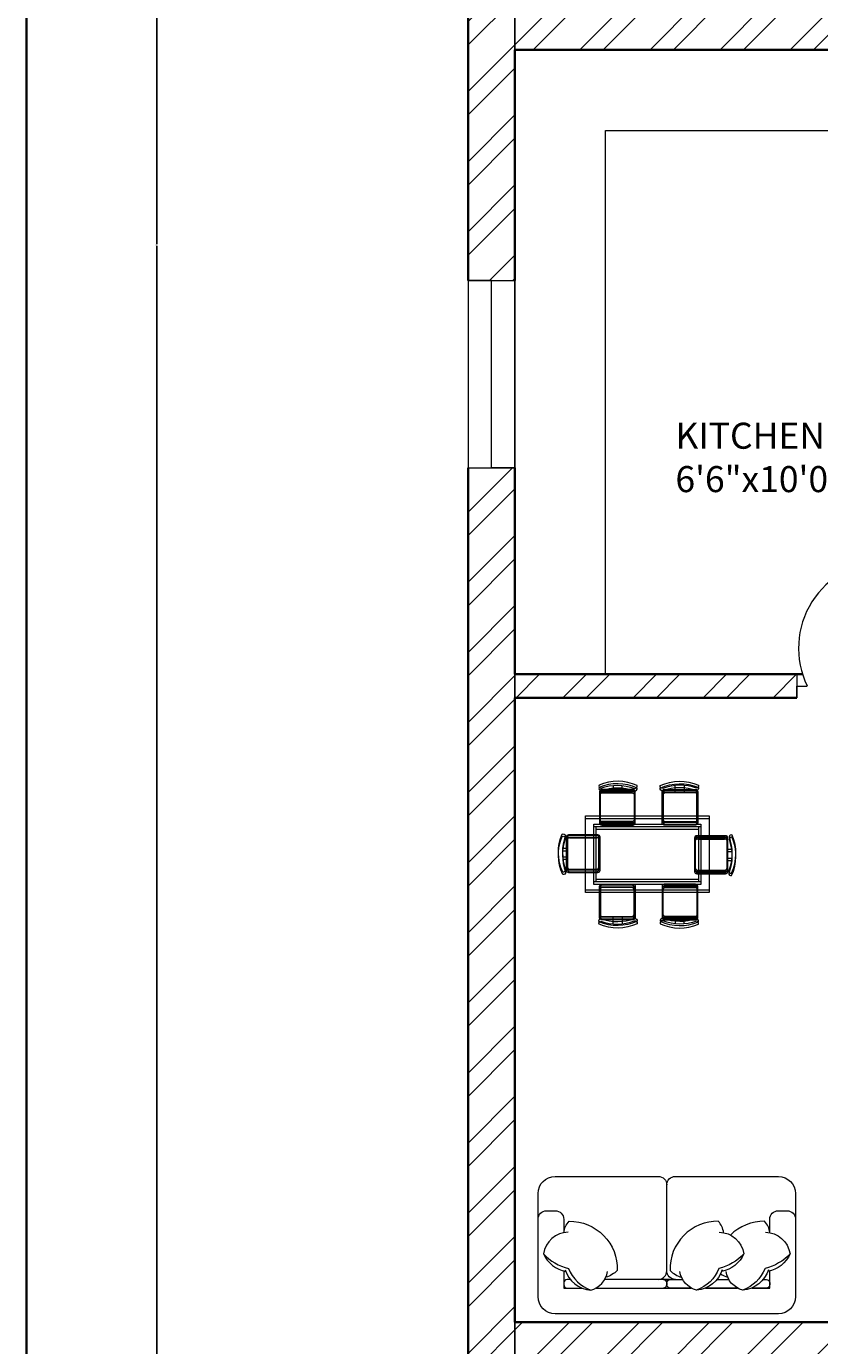
# Model space of a CAD drawing. Units: inches. Extents: x 2552 to 3217, y 1417 to 2737.
# Tile 7 of 25: x 2552 to 2705, y 1885 to 2138. Entities that reach past the tile are written whole.
import ezdxf

# ---------------------------------------------------------------- set-up
doc = ezdxf.new("R2010")
doc.units = ezdxf.units.IN
for name, color, linetype, lineweight in [('A-ANNO-DIMS', 2, 'Continuous', 18), ('A-ANNO-TTLB', 7, 'Continuous', 35), ('A-AREA-IDEN', 7, 'Continuous', 18), ('A-DOOR', 21, 'Continuous', 18), ('A-FLOR-CASE', 9, 'Continuous', 18), ('A-FURN', 8, 'Continuous', 13), ('A-GLAZ', 161, 'Continuous', 18), ('A-WALL', 7, 'Continuous', 35), ('A-WALL-PATT', 217, 'Continuous', 13)]:
    doc.layers.add(name, color=color, linetype=linetype, lineweight=lineweight)
doc.styles.get("Standard").update_dxf_attribs({"font": 'arial.ttf'})
doc.dimstyles.get("Standard").update_dxf_attribs({"dimtxt": 0.18, "dimasz": 0.18, "dimexe": 0.18, "dimexo": 0.0625, "dimgap": 0.09, "dimtad": 0, "dimtih": 1, "dimtoh": 1, "dimdec": 4, "dimzin": 0, "dimdsep": 46, "dimtxsty": 'Standard', "dimcen": 0.09, "dimadec": 0, "dimazin": 0, "dimtfac": 1, "dimtdec": 4, "dimtofl": 0, "dimtmove": 0, "dimatfit": 3, "dimfxl": 1, "dimtolj": 1, "dimtzin": 0, "dimarcsym": 0})

# ---------------------------------------------------------------- blocks, each defined once
blk = doc.blocks.new('DINING-SET-SIX')
for points in [[(8.15, 26.89, -0.175809), (14.62, 26.84, 0.578392), (15.11, 27.38, 0.214524), (7.8, 27.47, 0.552014), (8.15, 26.89, -0.065079)], [(8.15, 26.89, -0.175809), (14.62, 26.84, 0.578392), (15.11, 27.38, 0.214524), (7.8, 27.47, 0.552014), (8.15, 26.89, -0.065079)], [(20.07, 26.84, -0.578392), (19.58, 27.38, -0.214524), (26.89, 27.47, -0.552014), (26.55, 26.89, 0.175809), (20.07, 26.84)], [(20.07, 26.84, -0.578392), (19.58, 27.38, -0.214524), (26.89, 27.47, -0.552014), (26.55, 26.89, 0.175809), (20.07, 26.84)], [(8.15, 26.41, -0.175809), (14.62, 26.36, 0.578392), (15.11, 26.9, 0.214524), (7.8, 27, 0.552014), (8.15, 26.41, -0.065079)], [(8.15, 26.41, -0.175809), (14.62, 26.36, 0.578392), (15.11, 26.9, 0.214524), (7.8, 27, 0.552014), (8.15, 26.41, -0.065079)], [(14.35, 26.63), (8.33, 26.63, 0.414214), (7.91, 26.21), (7.91, 20.68, 0.414214), (8.33, 20.26), (14.35, 20.26, 0.414214), (14.77, 20.68), (14.77, 26.21, 0.414214), (14.35, 26.63)], [(14.35, 26.63), (8.33, 26.63, 0.414214), (7.91, 26.21), (7.91, 20.68, 0.414214), (8.33, 20.26), (14.35, 20.26, 0.414214), (14.77, 20.68), (14.77, 26.21, 0.414214), (14.35, 26.63)], [(14.35, 26.15), (8.33, 26.15, 0.414214), (7.91, 25.73), (7.91, 20.2, 0.414214), (8.33, 19.78), (14.35, 19.78, 0.414214), (14.77, 20.2), (14.77, 25.73, 0.414214), (14.35, 26.15)], [(14.35, 26.15), (8.33, 26.15, 0.414214), (7.91, 25.73), (7.91, 20.2, 0.414214), (8.33, 19.78), (14.35, 19.78, 0.414214), (14.77, 20.2), (14.77, 25.73, 0.414214), (14.35, 26.15)], [(12.23, 26.63), (12.23, 27.39, -0.064759)], [(12.23, 26.63), (12.23, 27.39, -0.064759)], [(12.23, 26.15), (12.23, 26.91, -0.064759)], [(12.23, 26.15), (12.23, 26.91, -0.064759)], [(20.07, 26.36, -0.578392), (19.58, 26.9, -0.214524), (26.89, 27, -0.552014), (26.55, 26.41, 0.175809), (20.07, 26.36)], [(20.07, 26.36, -0.578392), (19.58, 26.9, -0.214524), (26.89, 27, -0.552014), (26.55, 26.41, 0.175809), (20.07, 26.36)], [(26.36, 26.63, -0.414214), (26.78, 26.21), (26.78, 20.68, -0.414214), (26.36, 20.26), (20.35, 20.26, -0.414214), (19.92, 20.68), (19.92, 26.21, -0.414214), (20.35, 26.63), (26.36, 26.63)], [(26.36, 26.63, -0.414214), (26.78, 26.21), (26.78, 20.68, -0.414214), (26.36, 20.26), (20.35, 20.26, -0.414214), (19.92, 20.68), (19.92, 26.21, -0.414214), (20.35, 26.63), (26.36, 26.63)], [(26.36, 26.15, -0.414214), (26.78, 25.73), (26.78, 20.2, -0.414214), (26.36, 19.78), (20.35, 19.78, -0.414214), (19.92, 20.2), (19.92, 25.73, -0.414214), (20.35, 26.15), (26.36, 26.15)], [(26.36, 26.15, -0.414214), (26.78, 25.73), (26.78, 20.2, -0.414214), (26.36, 19.78), (20.35, 19.78, -0.414214), (19.92, 20.2), (19.92, 25.73, -0.414214), (20.35, 26.15), (26.36, 26.15)], [(22.46, 26.63), (22.46, 27.39, 0.064759)], [(22.46, 26.63), (22.46, 27.39, 0.064759)], [(22.46, 26.15), (22.46, 26.91, 0.064759)], [(22.46, 26.15), (22.46, 26.91, 0.064759)], [(1.37, 11.25, -0.578392), (0.83, 10.76, -0.214524), (0.73, 18.07, -0.552014), (1.32, 17.73, 0.175809), (1.37, 11.25)], [(1.37, 11.25, -0.578392), (0.83, 10.76, -0.214524), (0.73, 18.07, -0.552014), (1.32, 17.73, 0.175809), (1.37, 11.25)], [(1.58, 17.54, -0.414214), (2, 17.96), (7.53, 17.96, -0.414214), (7.95, 17.54), (7.95, 11.53, -0.414214), (7.53, 11.11), (2, 11.11, -0.414214), (1.58, 11.53), (1.58, 17.54)], [(1.58, 17.54, -0.414214), (2, 17.96), (7.53, 17.96, -0.414214), (7.95, 17.54), (7.95, 11.53, -0.414214), (7.53, 11.11), (2, 11.11, -0.414214), (1.58, 11.53), (1.58, 17.54)], [(32.54, 17.33, 0.414214), (32.11, 17.75), (26.59, 17.75, 0.414214), (26.17, 17.33), (26.17, 11.32, 0.414214), (26.59, 10.9), (32.11, 10.9, 0.414214), (32.54, 11.32), (32.54, 17.33)], [(32.54, 17.33, 0.414214), (32.11, 17.75), (26.59, 17.75, 0.414214), (26.17, 17.33), (26.17, 11.32, 0.414214), (26.59, 10.9), (32.11, 10.9, 0.414214), (32.54, 11.32), (32.54, 17.33)], [(32.79, 17.52, -0.175809), (32.75, 11.05, 0.578392), (33.29, 10.56, 0.214524), (33.38, 17.86, 0.552014), (32.79, 17.52, -0.065079)], [(32.79, 17.52, -0.175809), (32.75, 11.05, 0.578392), (33.29, 10.56, 0.214524), (33.38, 17.86, 0.552014), (32.79, 17.52, -0.065079)], [(1.37, 10.78, -0.578392), (0.83, 10.29, -0.214524), (0.73, 17.59, -0.552014), (1.32, 17.25, 0.175809), (1.37, 10.78)], [(1.37, 10.78, -0.578392), (0.83, 10.29, -0.214524), (0.73, 17.59, -0.552014), (1.32, 17.25, 0.175809), (1.37, 10.78)], [(1.58, 17.06, -0.414214), (2, 17.48), (7.53, 17.48, -0.414214), (7.95, 17.06), (7.95, 11.05, -0.414214), (7.53, 10.63), (2, 10.63, -0.414214), (1.58, 11.05), (1.58, 17.06)], [(1.58, 17.06, -0.414214), (2, 17.48), (7.53, 17.48, -0.414214), (7.95, 17.06), (7.95, 11.05, -0.414214), (7.53, 10.63), (2, 10.63, -0.414214), (1.58, 11.05), (1.58, 17.06)], [(32.54, 16.86, 0.414214), (32.11, 17.28), (26.59, 17.28, 0.414214), (26.17, 16.86), (26.17, 10.85, 0.414214), (26.59, 10.42), (32.11, 10.42, 0.414214), (32.54, 10.85), (32.54, 16.86)], [(32.54, 16.86, 0.414214), (32.11, 17.28), (26.59, 17.28, 0.414214), (26.17, 16.86), (26.17, 10.84, 0.414214), (26.59, 10.42), (32.11, 10.42, 0.414214), (32.54, 10.84), (32.54, 16.86)], [(32.79, 17.04, -0.175809), (32.75, 10.57, 0.578392), (33.29, 10.08, 0.214524), (33.38, 17.39, 0.552014), (32.79, 17.04, -0.065079)], [(32.79, 17.04, -0.175809), (32.75, 10.57, 0.578392), (33.29, 10.08, 0.214524), (33.38, 17.39, 0.552014), (32.79, 17.04, -0.065079)], [(1.58, 13.64), (0.82, 13.64, 0.064759)], [(1.58, 13.64), (0.82, 13.64, 0.064759)], [(1.58, 13.16), (0.82, 13.16, 0.064759)], [(1.58, 13.16), (0.82, 13.16, 0.064759)], [(32.54, 13.43), (33.3, 13.43, -0.064759)], [(32.54, 13.43), (33.3, 13.43, -0.064759)], [(32.54, 12.96), (33.3, 12.96, -0.064759)], [(32.54, 12.96), (33.3, 12.96, -0.064759)], [(14.35, 2.06), (8.33, 2.06, -0.414214), (7.91, 2.48), (7.91, 8.01, -0.414214), (8.33, 8.43), (14.35, 8.43, -0.414214), (14.77, 8.01), (14.77, 2.48, -0.414214), (14.35, 2.06)], [(14.35, 2.06), (8.33, 2.06, -0.414214), (7.91, 2.48), (7.91, 8.01, -0.414214), (8.33, 8.43), (14.35, 8.43, -0.414214), (14.77, 8.01), (14.77, 2.48, -0.414214), (14.35, 2.06)], [(14.35, 1.58), (8.33, 1.58, -0.414214), (7.91, 2), (7.91, 7.53, -0.414214), (8.33, 7.95), (14.35, 7.95, -0.414214), (14.77, 7.53), (14.77, 2, -0.414214), (14.35, 1.58)], [(14.35, 1.58), (8.33, 1.58, -0.414214), (7.91, 2), (7.91, 7.53, -0.414214), (8.33, 7.95), (14.35, 7.95, -0.414214), (14.77, 7.53), (14.77, 2, -0.414214), (14.35, 1.58)], [(26.36, 2.06, 0.414214), (26.78, 2.48), (26.78, 8.01, 0.414214), (26.36, 8.43), (20.35, 8.43, 0.414214), (19.92, 8.01), (19.92, 2.48, 0.414214), (20.35, 2.06), (26.36, 2.06)], [(26.36, 2.06, 0.414214), (26.78, 2.48), (26.78, 8.01, 0.414214), (26.36, 8.43), (20.35, 8.43, 0.414214), (19.92, 8.01), (19.92, 2.48, 0.414214), (20.35, 2.06), (26.36, 2.06)], [(26.36, 1.58, 0.414214), (26.78, 2), (26.78, 7.53, 0.414214), (26.36, 7.95), (20.35, 7.95, 0.414214), (19.92, 7.53), (19.92, 2, 0.414214), (20.35, 1.58), (26.36, 1.58)], [(26.36, 1.58, 0.414214), (26.78, 2), (26.78, 7.53, 0.414214), (26.36, 7.95), (20.35, 7.95, 0.414214), (19.92, 7.53), (19.92, 2, 0.414214), (20.35, 1.58), (26.36, 1.58)], [(14.62, 1.85, -0.578392), (15.11, 1.31, -0.214524), (7.8, 1.21, -0.552014), (8.15, 1.8, 0.175809), (14.62, 1.85)], [(14.62, 1.85, -0.578392), (15.11, 1.31, -0.214524), (7.8, 1.21, -0.552014), (8.15, 1.8, 0.175809), (14.62, 1.85)], [(14.62, 1.37, -0.578392), (15.11, 0.83, -0.214524), (7.8, 0.74, -0.552014), (8.15, 1.32, 0.175809), (14.62, 1.37)], [(14.62, 1.37, -0.578392), (15.11, 0.83, -0.214524), (7.8, 0.74, -0.552014), (8.15, 1.32, 0.175809), (14.62, 1.37)], [(12.23, 2.06), (12.23, 1.3, 0.064759)], [(12.23, 2.06), (12.23, 1.3, 0.064759)], [(12.23, 1.58), (12.23, 0.82, 0.064759)], [(12.23, 1.58), (12.23, 0.82, 0.064759)], [(26.55, 1.8, -0.175809), (20.07, 1.85, 0.578392), (19.58, 1.31, 0.214524), (26.89, 1.21, 0.552014), (26.55, 1.8, -0.065079)], [(26.55, 1.8, -0.175809), (20.07, 1.85, 0.578392), (19.58, 1.31, 0.214524), (26.89, 1.21, 0.552014), (26.55, 1.8, -0.065079)], [(26.55, 1.32, -0.175809), (20.07, 1.37, 0.578392), (19.58, 0.83, 0.214524), (26.89, 0.74, 0.552014), (26.55, 1.32, -0.065079)], [(26.55, 1.32, -0.175809), (20.07, 1.37, 0.578392), (19.58, 0.83, 0.214524), (26.89, 0.74, 0.552014), (26.55, 1.32, -0.065079)], [(22.46, 2.06), (22.46, 1.3, -0.064759)], [(22.46, 2.06), (22.46, 1.3, -0.064759)], [(22.46, 1.58), (22.46, 0.82, -0.064759)], [(22.46, 1.58), (22.46, 0.82, -0.064759)]]:
    blk.add_lwpolyline(points, format="xyb")
for points in [[(8.34, 26.44), (14.16, 26.44, -0.414214), (14.58, 26.02), (14.58, 20.87, -0.414214), (14.16, 20.45), (8.34, 20.45, -0.512069), (8.1, 20.87), (8.1, 26.02, -0.512069)], [(8.34, 26.44), (14.16, 26.44, -0.414214), (14.58, 26.02), (14.58, 20.87, -0.414214), (14.16, 20.45), (8.34, 20.45, -0.512069), (8.1, 20.87), (8.1, 26.02, -0.512069)], [(8.34, 25.96), (14.16, 25.96, -0.414214), (14.58, 25.54), (14.58, 20.39, -0.414214), (14.16, 19.97), (8.34, 19.97, -0.512069), (8.1, 20.39), (8.1, 25.54, -0.512069)], [(8.34, 25.96), (14.16, 25.96, -0.414214), (14.58, 25.54), (14.58, 20.39, -0.414214), (14.16, 19.97), (8.34, 19.97, -0.512069), (8.1, 20.39), (8.1, 25.54, -0.512069)], [(26.35, 26.44), (20.53, 26.44, 0.414214), (20.11, 26.02), (20.11, 20.87, 0.414214), (20.53, 20.45), (26.35, 20.45, 0.512069), (26.59, 20.87), (26.59, 26.02, 0.512069)], [(26.35, 26.44), (20.53, 26.44, 0.414214), (20.11, 26.02), (20.11, 20.87, 0.414214), (20.53, 20.45), (26.35, 20.45, 0.512069), (26.59, 20.87), (26.59, 26.02, 0.512069)], [(26.35, 25.96), (20.53, 25.96, 0.414214), (20.11, 25.54), (20.11, 20.39, 0.414214), (20.53, 19.97), (26.35, 19.97, 0.512069), (26.59, 20.39), (26.59, 25.54, 0.512069)], [(26.35, 25.96), (20.53, 25.96, 0.414214), (20.11, 25.54), (20.11, 20.39, 0.414214), (20.53, 19.97), (26.35, 19.97, 0.512069), (26.59, 20.39), (26.59, 25.54, 0.512069)], [(1.77, 17.53), (1.77, 11.72, 0.414214), (2.19, 11.3), (7.34, 11.3, 0.414214), (7.76, 11.72), (7.76, 17.53, 0.512069), (7.34, 17.77), (2.19, 17.77, 0.512069)], [(1.77, 17.53), (1.77, 11.72, 0.414214), (2.19, 11.29), (7.34, 11.29, 0.414214), (7.76, 11.72), (7.76, 17.53, 0.512069), (7.34, 17.77), (2.19, 17.77, 0.512069)], [(1.77, 17.06), (1.77, 11.24, 0.414214), (2.19, 10.82), (7.34, 10.82, 0.414214), (7.76, 11.24), (7.76, 17.06, 0.512069), (7.34, 17.29), (2.19, 17.29, 0.512069)], [(1.77, 17.06), (1.77, 11.24, 0.414214), (2.19, 10.82), (7.34, 10.82, 0.414214), (7.76, 11.24), (7.76, 17.06, 0.512069), (7.34, 17.29), (2.19, 17.29, 0.512069)], [(32.35, 17.33), (32.35, 11.51, -0.414214), (31.93, 11.09), (26.78, 11.09, -0.414214), (26.36, 11.51), (26.36, 17.33, -0.512069), (26.78, 17.56), (31.93, 17.56, -0.512069)], [(32.35, 17.33), (32.35, 11.51, -0.414214), (31.93, 11.09), (26.78, 11.09, -0.414214), (26.36, 11.51), (26.36, 17.33, -0.512069), (26.78, 17.56), (31.93, 17.56, -0.512069)], [(32.35, 16.85), (32.35, 11.03, -0.414214), (31.93, 10.61), (26.78, 10.61, -0.414214), (26.36, 11.03), (26.36, 16.85, -0.512069), (26.78, 17.09), (31.93, 17.09, -0.512069)], [(32.35, 16.85), (32.35, 11.03, -0.414214), (31.93, 10.61), (26.78, 10.61, -0.414214), (26.36, 11.03), (26.36, 16.85, -0.512069), (26.78, 17.09), (31.93, 17.09, -0.512069)], [(8.34, 2.25), (14.16, 2.25, 0.414214), (14.58, 2.67), (14.58, 7.82, 0.414214), (14.16, 8.24), (8.34, 8.24, 0.512069), (8.1, 7.82), (8.1, 2.67, 0.512069)], [(8.34, 2.25), (14.16, 2.25, 0.414214), (14.58, 2.67), (14.58, 7.82, 0.414214), (14.16, 8.24), (8.34, 8.24, 0.512069), (8.1, 7.82), (8.1, 2.67, 0.512069)], [(8.34, 1.77), (14.16, 1.77, 0.414214), (14.58, 2.19), (14.58, 7.34, 0.414214), (14.16, 7.76), (8.34, 7.76, 0.512069), (8.1, 7.34), (8.1, 2.19, 0.512069)], [(8.34, 1.77), (14.16, 1.77, 0.414214), (14.58, 2.19), (14.58, 7.34, 0.414214), (14.16, 7.76), (8.34, 7.76, 0.512069), (8.1, 7.34), (8.1, 2.19, 0.512069)], [(26.35, 2.25), (20.53, 2.25, -0.414214), (20.11, 2.67), (20.11, 7.82, -0.414214), (20.53, 8.24), (26.35, 8.24, -0.512069), (26.59, 7.82), (26.59, 2.67, -0.512069)], [(26.35, 2.25), (20.53, 2.25, -0.414214), (20.11, 2.67), (20.11, 7.82, -0.414214), (20.53, 8.24), (26.35, 8.24, -0.512069), (26.59, 7.82), (26.59, 2.67, -0.512069)], [(26.35, 1.77), (20.53, 1.77, -0.414214), (20.11, 2.19), (20.11, 7.34, -0.414214), (20.53, 7.76), (26.35, 7.76, -0.512069), (26.59, 7.34), (26.59, 2.19, -0.512069)], [(26.35, 1.77), (20.53, 1.77, -0.414214), (20.11, 2.19), (20.11, 7.34, -0.414214), (20.53, 7.76), (26.35, 7.76, -0.512069), (26.59, 7.34), (26.59, 2.19, -0.512069)]]:
    blk.add_lwpolyline(points, format="xyb", close=True)
for points in [[(10.55, 27.4), (10.55, 26.63)], [(10.55, 27.4), (10.55, 26.63)], [(10.55, 26.93), (10.55, 26.15)], [(10.55, 26.92), (10.55, 26.15)], [(24.14, 27.4), (24.14, 26.63)], [(24.14, 27.4), (24.14, 26.63)], [(24.14, 26.93), (24.14, 26.15)], [(24.14, 26.92), (24.14, 26.15)], [(0.81, 15.32), (1.58, 15.32)], [(0.81, 15.32), (1.58, 15.32)], [(0.81, 14.84), (1.58, 14.84)], [(0.81, 14.84), (1.58, 14.84)], [(33.31, 15.11), (32.54, 15.11)], [(33.31, 15.11), (32.54, 15.11)], [(33.31, 14.64), (32.54, 14.64)], [(33.31, 14.64), (32.54, 14.64)], [(10.55, 1.29), (10.55, 2.06)], [(10.55, 1.28), (10.55, 2.06)], [(10.55, 0.81), (10.55, 1.58)], [(10.55, 0.81), (10.55, 1.58)], [(24.14, 1.29), (24.14, 2.06)], [(24.14, 1.28), (24.14, 2.06)], [(24.14, 0.81), (24.14, 1.58)], [(24.14, 0.81), (24.14, 1.58)]]:
    blk.add_lwpolyline(points)
for points in [[(5.21, 21.55), (28.98, 21.55), (28.98, 7.29), (5.21, 7.29)], [(5.21, 21.55), (28.98, 21.55), (28.98, 7.29), (5.21, 7.29)], [(5.21, 21.08), (28.98, 21.08), (28.98, 6.81), (5.21, 6.81)], [(5.21, 21.07), (28.98, 21.07), (28.98, 6.81), (5.21, 6.81)], [(6.79, 19.97), (27.39, 19.97), (27.39, 8.87), (6.79, 8.87)], [(6.79, 19.97), (27.39, 19.97), (27.39, 8.87), (6.79, 8.87)], [(6.79, 19.49), (27.39, 19.49), (27.39, 8.4), (6.79, 8.4)], [(6.79, 19.49), (27.39, 19.49), (27.39, 8.4), (6.79, 8.4)], [(7.27, 19.49), (26.92, 19.49), (26.92, 9.35), (7.27, 9.35)], [(7.27, 19.49), (26.92, 19.49), (26.92, 9.35), (7.27, 9.35)], [(7.27, 19.01), (26.92, 19.01), (26.92, 8.87), (7.27, 8.87)], [(7.27, 19.01), (26.92, 19.01), (26.92, 8.87), (7.27, 8.87)]]:
    blk.add_lwpolyline(points, close=True)
blk = doc.blocks.new('WIN-36')
for p, q in [((4.5, 36), (0, 36)), ((0, 36), (9, 36)), ((0, 36), (0, 0)), ((4.5, 0), (4.5, 36)), ((9, 36), (9, 0)), ((0, 0), (9, 0)), ((9, 0), (4.5, 0))]:
    blk.add_line(p, q)
blk = doc.blocks.new('*D50')
at = {"layer": 'A-ANNO-DIMS', "color": 0, "lineweight": -2, "transparency": 16777216}
for p, q in [((2637.29, 2649.51), (2577.37, 2649.51)), ((2577.55, 2649.33), (2577.55, 2096.19)), ((2577.55, 1542.69), (2577.55, 2095.83)), ((2637.29, 1542.51), (2577.37, 1542.51))]:
    blk.add_line(p, q, dxfattribs=at)
at = {"layer": 'A-ANNO-DIMS', "color": 0, "transparency": 16777216}
for points in [[(2577.52, 2649.33), (2577.58, 2649.33), (2577.55, 2649.51)], [(2577.52, 1542.69), (2577.58, 1542.69), (2577.55, 1542.51)]]:
    blk.add_solid(points, dxfattribs=at)
at = {"layer": 'Defpoints', "color": 0, "transparency": 16777216}
for p in [(2577.55, 2649.51), (2637.35, 2649.51), (2637.35, 1542.51)]:
    blk.add_point(p, dxfattribs=at)
at = {"layer": 'A-ANNO-DIMS', "color": 0, "transparency": 16777216, "insert": (2577.55, 2096.01), "char_height": 0.18, "attachment_point": 5}
blk.add_mtext('\\A1;1107', dxfattribs=at)
blk = doc.blocks.new('*D64')
at = {"layer": 'A-ANNO-DIMS', "color": 0, "lineweight": -2, "transparency": 16777216}
for p, q in [((2646.35, 1551.58), (2646.35, 2709.49)), ((2646.53, 2709.31), (2802.77, 2709.31)), ((2959.93, 2709.31), (2803.69, 2709.31)), ((2960.11, 1551.58), (2960.11, 2709.49))]:
    blk.add_line(p, q, dxfattribs=at)
at = {"layer": 'A-ANNO-DIMS', "color": 0, "transparency": 16777216}
for points in [[(2646.53, 2709.34), (2646.53, 2709.28), (2646.35, 2709.31)], [(2959.93, 2709.34), (2959.93, 2709.28), (2960.11, 2709.31)]]:
    blk.add_solid(points, dxfattribs=at)
at = {"layer": 'Defpoints', "color": 0, "transparency": 16777216}
for p in [(2960.11, 2709.31), (2646.35, 1551.51), (2960.11, 1551.51)]:
    blk.add_point(p, dxfattribs=at)
at = {"layer": 'A-ANNO-DIMS', "color": 0, "transparency": 16777216, "insert": (2803.23, 2709.31), "char_height": 0.18, "attachment_point": 5}
blk.add_mtext('\\A1;313.76', dxfattribs=at)

msp = doc.modelspace()

# ---------------------------------------------------------------- hatches: boundary and pattern name
at = {"layer": 'A-WALL-PATT'}
h = msp.add_hatch(dxfattribs=at)
h.set_pattern_fill('ANSI32', color=256)
h.paths.add_polyline_path([(2756.676, 2649.5125), (2637.3535, 2649.5125), (2637.3535, 2617.9626), (2641.8535, 2617.9626), (2646.3535, 2617.9626), (2646.3535, 2640.5125), (2724.3535, 2640.5125), (2724.3535, 2520.5125), (2720.299, 2520.5125), (2720.299, 2516.0125), (2733.4075, 2516.0125), (2733.4075, 2518.2213), (2733.4075, 2520.5125), (2728.8535, 2520.5125), (2728.8535, 2640.5125), (2756.676, 2640.5125)])
h.paths.add_polyline_path([(2848.8535, 2649.5125), (2804.676, 2649.5125), (2804.676, 2640.5125), (2839.8535, 2640.5125), (2839.8535, 2598.3517), (2848.8535, 2598.3517)])
h.paths.add_polyline_path([(2646.3535, 2516.0125), (2697.9593, 2516.0125), (2697.9593, 2518.2625), (2697.9593, 2520.5125), (2646.3535, 2520.5125), (2646.3535, 2581.9626), (2637.3535, 2581.9626), (2637.3535, 2364.3298), (2646.3535, 2364.3298), (2646.3535, 2387.0125), (2724.3535, 2387.0125), (2724.3535, 2267.0125), (2721.0443, 2267.0125), (2721.0443, 2262.5125), (2733.7854, 2262.5125), (2733.7854, 2264.7625), (2733.7854, 2267.0125), (2728.8535, 2267.0125), (2728.8535, 2387.0125), (2839.8535, 2387.0125), (2839.8535, 2363.8387), (2848.8535, 2363.8387), (2848.8535, 2403.7415), (2844.3535, 2403.7415), (2839.8535, 2403.7415), (2839.8535, 2396.0125), (2646.3535, 2396.0125)])
h.paths.add_polyline_path([(2848.8535, 2550.3517), (2844.3535, 2550.3517), (2839.8535, 2550.3517), (2839.8535, 2520.5125), (2801.9195, 2520.5125), (2801.9195, 2518.2625), (2801.9195, 2516.0125), (2839.8535, 2516.0125), (2839.8535, 2507.5813), (2848.8535, 2507.5813)], flags=17)
h.paths.add_polyline_path([(2848.8535, 2483.5813), (2844.3535, 2483.5813), (2839.8535, 2483.5813), (2839.8535, 2468.0125), (2773.8535, 2468.0125), (2773.8535, 2516.0125), (2778.1336, 2516.0125), (2778.1336, 2520.5125), (2766.696, 2520.5125), (2766.696, 2518.2625), (2766.696, 2516.0125), (2769.3535, 2516.0125), (2769.3535, 2463.5125), (2839.8535, 2463.5125), (2839.8535, 2431.0782), (2848.8535, 2431.0782)], flags=17)
h.paths.add_polyline_path([(2917.8535, 2569.2764), (2913.3535, 2569.2764), (2908.8535, 2569.2764), (2908.8535, 2433.001), (2917.8535, 2433.001), (2917.8535, 2516.0125), (2967.486, 2516.0125), (2967.486, 2520.5125), (2917.8535, 2520.5125)])
h.paths.add_polyline_path([(3000.3535, 2640.5125), (2995.8535, 2640.5125), (2995.8535, 2520.5125), (2990.688, 2520.5125), (2990.688, 2516.0125), (3004.0844, 2516.0125), (3004.0844, 2518.2625), (3004.0844, 2520.5125), (3000.3535, 2520.5125)])
h.paths.add_polyline_path([(3120.3535, 2561.3689), (3115.8535, 2561.3689), (3111.3535, 2561.3689), (3111.3535, 2520.5125), (3070.9814, 2520.5125), (3070.9814, 2518.2625), (3070.9814, 2516.0125), (3111.3535, 2516.0125), (3111.3535, 2505.1841), (3120.3535, 2505.1841)])
h.paths.add_polyline_path([(3120.3535, 2481.1841), (3115.8535, 2481.1841), (3111.3535, 2481.1841), (3111.3535, 2468.0125), (3045.3535, 2468.0125), (3045.3535, 2516.0125), (3048.9787, 2516.0125), (3048.9787, 2520.5125), (3036.3395, 2520.5125), (3036.3395, 2516.0125), (3040.8535, 2516.0125), (3040.8535, 2463.5125), (3111.3535, 2463.5125), (3111.3535, 2396.0125), (2917.8535, 2396.0125), (2917.8535, 2403.4124), (2913.3535, 2403.4124), (2908.8535, 2403.4124), (2908.8535, 2182.5756), (2917.8535, 2182.5756), (2917.8535, 2262.5125), (2968.001, 2262.5125), (2968.001, 2264.7625), (2968.001, 2267.0125), (2917.8535, 2267.0125), (2917.8535, 2387.0125), (3111.3535, 2387.0125), (3111.3535, 2352.2435), (3120.3535, 2352.2435)])
h.paths.add_polyline_path([(3120.3535, 2304.2435), (3115.8535, 2304.2435), (3111.3535, 2304.2435), (3111.3535, 2267.0125), (3073.8616, 2267.0125), (3073.8616, 2264.7625), (3073.8616, 2262.5125), (3111.3535, 2262.5125), (3111.3535, 2252.376), (3120.3535, 2252.376)], flags=17)
h.paths.add_polyline_path([(3120.3535, 2228.376), (3115.8535, 2228.376), (3111.3535, 2228.376), (3111.3535, 2214.5125), (3045.3535, 2214.5125), (3045.3535, 2262.5125), (3049.3096, 2262.5125), (3049.3096, 2267.0125), (3035.0125, 2267.0125), (3035.0125, 2262.5125), (3040.8535, 2262.5125), (3040.8535, 2210.0125), (3111.3535, 2210.0125), (3111.3535, 2142.5125), (2917.8535, 2142.5125), (2917.8535, 2150.2408), (2913.3535, 2150.2408), (2908.8535, 2150.2408), (2908.8535, 1924.9905), (2917.8535, 1924.9905), (2917.8535, 2009.0125), (2971.959, 2009.0125), (2971.959, 2011.2625), (2971.959, 2013.5125), (2917.8535, 2013.5125), (2917.8535, 2133.5125), (2995.8535, 2133.5125), (2995.8535, 2013.5125), (2992.1797, 2013.5125), (2992.1797, 2009.0125), (3004.3344, 2009.0125), (3004.3344, 2011.2625), (3004.3344, 2013.5125), (3000.3535, 2013.5125), (3000.3535, 2133.5125), (3111.3535, 2133.5125), (3111.3535, 2115.0291), (3120.3535, 2115.0291)])
h.paths.add_polyline_path([(3000.3535, 2387.0125), (2995.8535, 2387.0125), (2995.8535, 2267.0125), (2991.3326, 2267.0125), (2991.3326, 2262.5125), (3004.1044, 2262.5125), (3004.1044, 2264.7625), (3004.1044, 2267.0125), (3000.3535, 2267.0125)], flags=17)
h.paths.add_polyline_path([(3120.3535, 1973.2388), (3115.8535, 1973.2388), (3111.3535, 1973.2388), (3111.3535, 1961.0125), (3045.3535, 1961.0125), (3045.3535, 2009.0125), (3048.9101, 2009.0125), (3048.9101, 2013.5125), (3037.105, 2013.5125), (3037.105, 2011.2625), (3037.105, 2009.0125), (3040.8535, 2009.0125), (3040.8535, 1956.5125), (3111.3535, 1956.5125), (3111.3535, 1889.0125), (2917.8535, 1889.0125), (2917.8535, 1895.7215), (2913.3535, 1895.7215), (2908.8535, 1895.7215), (2908.8535, 1844.2217), (2917.8535, 1844.2217), (2917.8535, 1880.0125), (3111.3535, 1880.0125), (3111.3535, 1846.9541), (3120.3535, 1846.9541)])
h.paths.add_polyline_path([(3120.3535, 2067.0291), (3111.3535, 2067.0291), (3111.3535, 2013.5125), (3071.3001, 2013.5125), (3071.3001, 2009.0125), (3111.3535, 2009.0125), (3111.3535, 1997.2388), (3120.3535, 1997.2388)], flags=0)
h.paths.add_polyline_path([(3120.3535, 1798.9541), (3115.8535, 1798.9541), (3111.3535, 1798.9541), (3111.3535, 1760.0125), (3071.2497, 1760.0125), (3071.2497, 1757.7625), (3071.2497, 1755.5125), (3111.3535, 1755.5125), (3111.3535, 1746.162), (3120.3535, 1746.2478)])
h.paths.add_polyline_path([(3120.3535, 1722.2049), (3111.3535, 1722.2049), (3111.3535, 1707.5125), (3045.3535, 1707.5125), (3045.3535, 1755.5125), (3048.6624, 1755.5125), (3048.6624, 1760.0125), (3035.3703, 1760.0125), (3035.3703, 1755.5125), (3040.8535, 1755.5125), (3040.8535, 1703.0125), (3111.3535, 1703.0125), (3111.3535, 1635.5125), (2917.8535, 1635.5125), (2917.8535, 1643.1366), (2913.3535, 1643.1366), (2908.8535, 1643.1366), (2908.8535, 1626.5125), (3120.3535, 1626.5125)])
h.paths.add_polyline_path([(2917.8535, 1755.5125), (2973.2287, 1755.5125), (2973.2287, 1757.7625), (2973.2287, 1760.0125), (2917.8535, 1760.0125), (2917.8535, 1808.2217), (2913.3535, 1808.2217), (2908.8535, 1808.2217), (2908.8535, 1676.1665), (2917.8535, 1676.1665)])
h.paths.add_polyline_path([(3000.3535, 1880.0125), (2995.8535, 1880.0125), (2995.8535, 1760.0125), (2992.9329, 1760.0125), (2992.9329, 1755.5125), (3003.8766, 1755.5125), (3003.8766, 1757.7625), (3003.8766, 1760.0125), (3000.3535, 1760.0125)])
h.paths.add_polyline_path([(2848.8535, 1896.6971), (2844.3535, 1896.6971), (2839.8535, 1896.6971), (2839.8535, 1889.0125), (2646.3535, 1889.0125), (2646.3535, 2009.0125), (2700.5253, 2009.0125), (2700.5253, 2011.2625), (2700.5253, 2013.5125), (2646.3535, 2013.5125), (2646.3535, 2053.1812), (2641.8535, 2053.1812), (2637.3535, 2053.1812), (2637.3535, 1836.254), (2646.3535, 1836.254), (2646.3535, 1880.0125), (2724.3535, 1880.0125), (2724.3535, 1760.0125), (2721.2473, 1760.0125), (2721.2473, 1755.5125), (2731.9187, 1755.5125), (2731.9187, 1757.7625), (2731.9187, 1760.0125), (2728.8535, 1760.0125), (2728.8535, 1880.0125), (2839.8535, 1880.0125), (2839.8535, 1840.3813), (2848.8535, 1840.3813)])
h.paths.add_polyline_path([(2848.8535, 1792.3813), (2844.3535, 1792.3813), (2839.8535, 1792.3813), (2839.8535, 1760.0125), (2797.8845, 1760.0125), (2797.8845, 1755.5125), (2839.8535, 1755.5125), (2839.8535, 1743.3688), (2844.3535, 1743.3688), (2848.8535, 1743.3688)], flags=0)
h.paths.add_polyline_path([(2848.8535, 1719.3688), (2844.3535, 1719.3688), (2839.8535, 1719.3688), (2839.8535, 1707.5125), (2773.8535, 1707.5125), (2773.8535, 1755.5125), (2777.716, 1755.5125), (2777.716, 1760.0125), (2760.9247, 1760.0125), (2760.9247, 1757.9721), (2760.9247, 1755.5125), (2769.3535, 1755.5125), (2769.3535, 1703.0125), (2839.8535, 1703.0125), (2839.8535, 1673.0277), (2848.8535, 1672.9407)], flags=0)
h.paths.add_polyline_path([(2646.3535, 1755.5125), (2702.9171, 1755.5125), (2702.9171, 1757.7625), (2702.9171, 1760.0125), (2646.3535, 1760.0125), (2646.3535, 1800.254), (2641.8535, 1800.254), (2637.3535, 1800.254), (2637.3535, 1626.5125), (2848.8535, 1626.5125), (2848.8535, 1643.1187), (2844.3535, 1643.1187), (2839.8535, 1643.1187), (2839.8535, 1635.5125), (2646.3535, 1635.5125)])
h.paths.add_polyline_path([(2848.8535, 2148.8427), (2844.3535, 2148.8427), (2839.8535, 2148.8427), (2839.8535, 2142.5125), (2646.3535, 2142.5125), (2646.3535, 2262.5125), (2701.3562, 2262.5125), (2701.3562, 2264.7625), (2701.3562, 2267.0125), (2646.3535, 2267.0125), (2646.3535, 2328.3298), (2637.3535, 2328.3298), (2637.3535, 2089.1812), (2646.3535, 2089.1812), (2646.3535, 2133.5125), (2839.8535, 2133.5125), (2839.8535, 2097.5966), (2848.8535, 2097.5966)])
h.paths.add_polyline_path([(2728.8535, 2133.5125), (2724.3535, 2133.5125), (2724.3535, 2013.5125), (2719.6039, 2013.5125), (2719.6039, 2009.0125), (2732.5784, 2009.0125), (2732.5784, 2011.2625), (2732.5784, 2013.5125), (2728.8535, 2013.5125)])
h.paths.add_polyline_path([(2848.8535, 1970.0557), (2844.3535, 1970.0557), (2839.8535, 1970.0557), (2839.8535, 1961.0125), (2773.8535, 1961.0125), (2773.8535, 2009.0125), (2777.3388, 2009.0125), (2777.3388, 2013.5125), (2764.7681, 2013.5125), (2764.7681, 2009.0125), (2769.3535, 2009.0125), (2769.3535, 1956.5125), (2839.8535, 1956.5125), (2839.8535, 1924.7199), (2848.8535, 1924.7199)], flags=17)
h.paths.add_polyline_path([(2848.8535, 2049.5966), (2844.3535, 2049.5966), (2839.8535, 2049.5966), (2839.8535, 2013.5125), (2798.198, 2013.5125), (2798.198, 2011.2625), (2798.198, 2009.0125), (2839.8535, 2009.0125), (2839.8535, 1994.0557), (2848.8535, 1994.0557)], flags=17)
h.paths.add_polyline_path([(2848.8535, 2315.8387), (2839.8535, 2315.8387), (2839.8535, 2267.0125), (2799.3375, 2267.0125), (2799.3375, 2264.7625), (2799.3375, 2262.5125), (2839.8535, 2262.5125), (2839.8535, 2253.2843), (2848.8535, 2253.2843)], flags=17)
h.paths.add_polyline_path([(2848.8535, 2229.2843), (2839.8535, 2229.2843), (2839.8535, 2177.6936), (2848.8535, 2177.6936)], flags=17)
h.paths.add_polyline_path([(2839.8535, 2214.5125), (2773.8535, 2214.5125), (2773.8535, 2262.5125), (2777.6984, 2262.5125), (2777.6984, 2267.0125), (2763.8226, 2267.0125), (2763.8226, 2262.5125), (2769.3535, 2262.5125), (2769.3535, 2210.0125), (2839.8535, 2210.0125)], flags=17)
h.paths.add_polyline_path([(3050.32, 2520.2817), (3088.9114, 2520.2817), (3088.9114, 2538.939), (3050.32, 2538.939)], flags=9)

# ---------------------------------------------------------------- linework, layer by layer
at = {"layer": 'A-ANNO-TTLB'}
msp.add_lwpolyline([(2552.473, 2736.5692), (3216.7862, 2736.5692), (3216.7862, 1416.6914), (2552.473, 1416.6914)], close=True, dxfattribs=at)
at = {"layer": 'A-DOOR'}
for p, q in [((2700.5253, 2013.5125), (2700.5253, 2009.0125)), ((2700.5253, 2009.0125), (2700.5253, 2011.2625)), ((2700.5253, 2011.2625), (2702.5253, 2011.2625))]:
    msp.add_line(p, q, dxfattribs=at)
msp.add_arc((2717.6039, 2018.5258), 16.7367, 90, 205.719887, dxfattribs=at)
at = {"layer": 'A-FLOR-CASE'}
for p, q in [((2663.7921, 2013.5125), (2663.7921, 2118.0143)), ((2663.7921, 2118.0143), (2724.3535, 2118.0143))]:
    msp.add_line(p, q, dxfattribs=at)
at = {"layer": 'A-FURN', "ltscale": 0.03}
msp.add_lwpolyline([(2673.8957, 1917.026, -0.41421356), (2675.5453, 1915.3765, -0.41421356), (2677.1949, 1917.026), (2696.9896, 1917.026, -0.41421356), (2700.2887, 1913.7269), (2700.2887, 1893.9321, -0.41421356), (2696.9896, 1890.633), (2654.101, 1890.633, -0.41421356), (2650.8018, 1893.9321), (2650.8018, 1913.7269, -0.41421356), (2654.101, 1917.026), (2673.8957, 1917.026, -0.41421356), (2675.5453, 1915.3765, -0.41421356), (2677.1949, 1917.026)], format="xyb", dxfattribs=at)
at = {"layer": 'A-FURN'}
for points in [[(2673.8957, 1897.2313, 0.41421356), (2675.5453, 1898.8808), (2675.5453, 1915.3765, 0.41421356)], [(2677.1949, 1897.2313, -0.41421356), (2675.5453, 1898.8808), (2675.5453, 1915.3765, -0.41421356)], [(2650.8018, 1908.7782, -0.41421356), (2652.4514, 1910.4278), (2654.101, 1910.4278, -0.41421356), (2655.7505, 1908.7782), (2655.7505, 1906.2224)], [(2695.3401, 1906.2224), (2695.3401, 1908.7782, -0.41421356), (2696.9896, 1910.4278), (2698.6392, 1910.4278, -0.41421356), (2700.2887, 1908.7782)], [(2656.5783, 1906.3223, 0.35677236), (2651.8517, 1902.1643, 0.24954205), (2656.1345, 1898.7379, -9.61688035)], [(2655.7469, 1906.2217, -0.16554063), (2656.7674, 1908.4012, -0.42598917), (2666.0317, 1898.9514, -0.12152332), (2663.8325, 1897.6489, 7.11546429)], [(2686.4575, 1906.2217, 0.16554063), (2685.437, 1908.4012, 0.42598917), (2676.1728, 1898.9514, 0.12152332), (2678.3719, 1897.6489, -7.11546429)], [(2685.6261, 1906.3223, -0.35677236), (2690.3528, 1902.1643, -0.24954205), (2686.07, 1898.7379, 9.61688035)], [(2695.3436, 1906.2217, 0.16554063), (2694.3232, 1908.4012, 0.20023115), (2687.775, 1905.7468, 0.12152332)], [(2694.5122, 1906.3223, -0.35677236), (2699.2389, 1902.1643, -0.24954205), (2694.9561, 1898.7379, 9.61688035)], [(2651.8517, 1902.1643, 0.14772988), (2656.6729, 1899.3294, 0.21334276), (2660.9269, 1895.1715, 0.17866181)], [(2690.3528, 1902.1643, -0.14772988), (2685.5316, 1899.3294, -0.21334276), (2681.2776, 1895.1715, -0.17866181)], [(2699.2389, 1902.1643, -0.14772988), (2694.4177, 1899.3294, -0.21334276), (2690.1637, 1895.1715, -0.17866181)], [(2656.0068, 1899.1035, 0.30666349), (2660.9269, 1895.1715, 0.30632997), (2664.141, 1898.7624, -0.87284716)], [(2673.8957, 1897.2313, 0.41421356), (2675.5453, 1898.8808)], [(2677.1949, 1897.2313, -0.41421356), (2675.5453, 1898.8808)], [(2686.1976, 1899.1035, -0.30666349), (2681.2776, 1895.1715, -0.30632997), (2678.0634, 1898.7624, 0.87284716)], [(2695.0838, 1899.1035, -0.30666349), (2690.1637, 1895.1715, -0.30632997), (2686.9496, 1898.7624, 0.87284716)], [(2691.8698, 1895.5817), (2695.3401, 1895.5817), (2695.3401, 1898.8235, -0.41421356)], [(2657.0093, 1897.2313), (2656.4104, 1897.2313, 0.41421356), (2655.7505, 1896.5714), (2655.7505, 1896.2415, 0.41421356), (2656.4104, 1895.5817)], [(2661.965, 1895.5817), (2674.8855, 1895.5817, 0.41421356), (2675.5453, 1896.2415), (2675.5453, 1896.5714, 0.41421356), (2674.8855, 1897.2313), (2663.626, 1897.2313, 0.41421356)], [(2680.2394, 1895.5817), (2676.2051, 1895.5817, -0.41421356), (2675.5453, 1896.2415), (2675.5453, 1896.5714, -0.41421356), (2676.2051, 1897.2313), (2678.5784, 1897.2313, -0.41421356)], [(2685.1951, 1897.2313), (2687.4645, 1897.2313, -0.41421356)], [(2685.8751, 1898.2938, 0.07186538), (2687.2581, 1897.6489, -7.11546429)], [(2694.0812, 1897.2313), (2694.6802, 1897.2313, -0.41421356), (2695.3401, 1896.5714), (2695.3401, 1896.2415, -0.41421356), (2694.6802, 1895.5817)], [(2656.4104, 1895.5817), (2659.2208, 1895.5817, 0.41421356)], [(2689.1256, 1895.5817), (2682.9837, 1895.5817, -0.41421356)], [(2694.6802, 1895.5817), (2691.8698, 1895.5817, -0.41421356)]]:
    msp.add_lwpolyline(points, format="xyb", dxfattribs=at)
for points in [[(2655.7505, 1898.8235), (2655.7505, 1895.5817), (2659.2208, 1895.5817)], [(2661.965, 1895.5817), (2680.2394, 1895.5817)], [(2682.9837, 1895.5817), (2689.1256, 1895.5817)]]:
    msp.add_lwpolyline(points, dxfattribs=at)
msp.add_lwpolyline([(2674.8855, 1895.5817), (2676.2051, 1895.5817, -0.41421356), (2675.5453, 1896.2415), (2675.5453, 1896.5714, -0.41421356), (2676.2051, 1897.2313), (2674.8855, 1897.2313, -0.41421356), (2675.5453, 1896.5714), (2675.5453, 1896.2415, -0.41421356)], format="xyb", close=True, dxfattribs=at)
at = {"layer": 'A-WALL'}
for p, q in [((2637.3535, 2328.3298), (2637.3535, 2089.1812)), ((2646.3535, 2133.5125), (2839.8535, 2133.5125)), ((2646.3535, 2133.5125), (2646.3535, 2089.1812)), ((2637.3535, 2053.1812), (2637.3535, 1836.254)), ((2646.3535, 2053.1812), (2646.3535, 2013.5125)), ((2646.3535, 2013.5125), (2701.6356, 2013.5125)), ((2646.3535, 2009.0125), (2700.5253, 2009.0125)), ((2646.3535, 2009.0125), (2646.3535, 1889.0125)), ((2646.3535, 1889.0125), (2839.8535, 1889.0125))]:
    msp.add_line(p, q, dxfattribs=at)

# ---------------------------------------------------------------- block references
at = {"layer": 'A-FURN'}
msp.add_blockref('DINING-SET-SIX', (2654.7197, 1964.7508), dxfattribs=at)
at = {"layer": 'A-GLAZ'}
msp.add_blockref('WIN-36', (2637.354, 2053.1815), dxfattribs=at)

# ---------------------------------------------------------------- texts
at = {"layer": 'A-AREA-IDEN', "insert": (2677.1982, 2061.8528), "char_height": 5, "attachment_point": 1}
msp.add_mtext_dynamic_manual_height_columns('KITCHEN\\P6\'6"x10\'0"', width=123.291199, gutter_width=12.5, heights=[0], dxfattribs=at)

# ---------------------------------------------------------------- dimensions: what is measured, and where the dimension line sits
at = {"layer": 'A-ANNO-DIMS'}
dim = msp.add_linear_dim(base=(2960.1089, 2709.3125), p1=(2646.3535, 1551.5125), p2=(2960.1089, 1551.5125), dimstyle='Standard', override={"dimdec": 2, "dimlfac": 1, "dimrnd": 0, "dimzin": 0, "dimdsep": 46, "dimlunit": 2}, dxfattribs=at)
dim.commit()
dim.dimension.update_dxf_attribs({"geometry": '*D64', "text_midpoint": (2803.2312, 2709.3125)})
dim = msp.add_linear_dim(base=(2577.5535, 2649.5125), p1=(2637.3535, 1542.5125), p2=(2637.3535, 2649.5125), angle=90, dimstyle='Standard', override={"dimdec": 0, "dimlfac": 1, "dimrnd": 0, "dimzin": 0, "dimdsep": 46, "dimlunit": 2}, dxfattribs=at)
dim.commit()
dim.dimension.update_dxf_attribs({"geometry": '*D50', "text_midpoint": (2577.5535, 2096.0125)})

doc.saveas('drawing.dxf')
